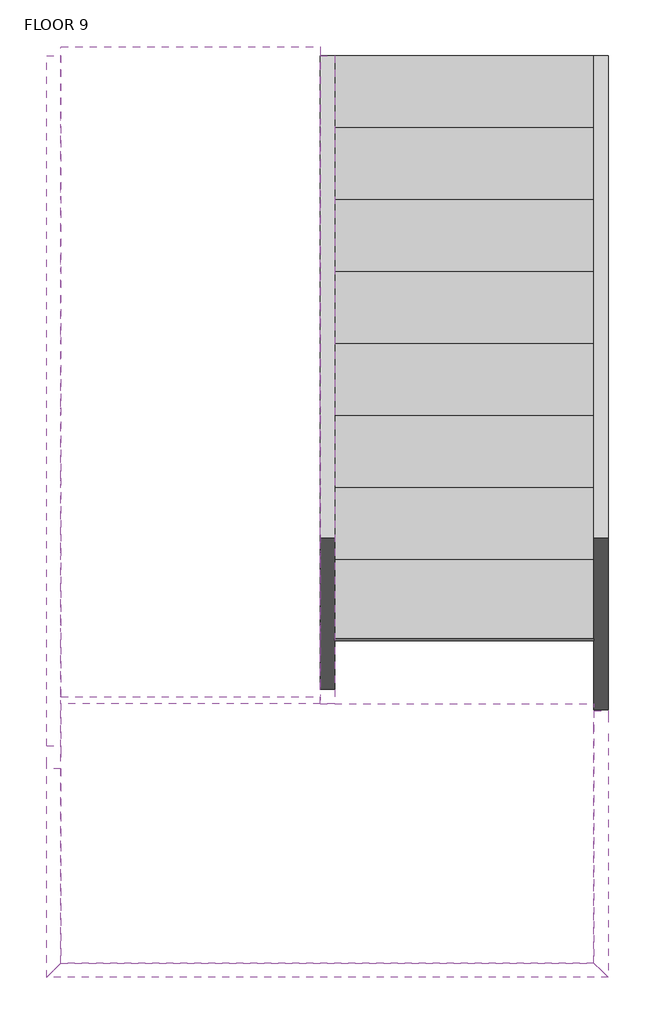
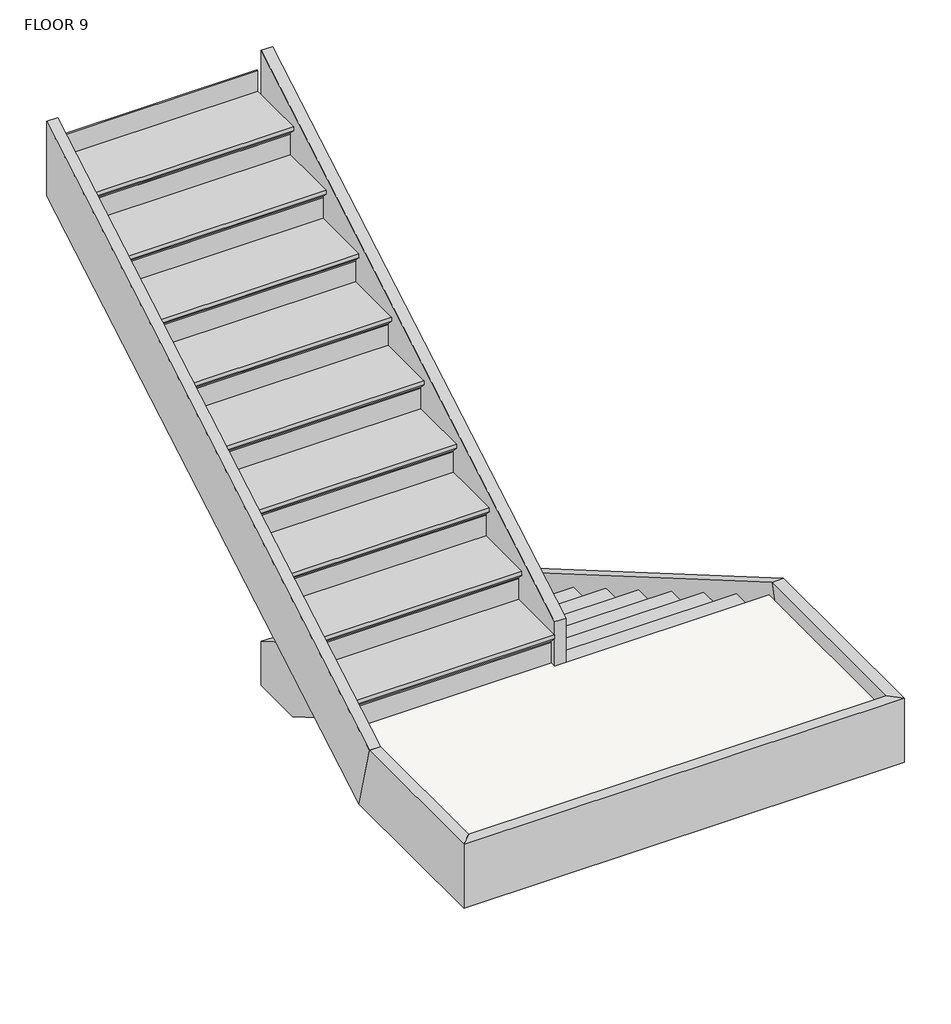
# One storey, incomplete: 7 members, 2 stair flights, 1 slab.
"""IFC4 building model written with IfcOpenShell, lengths in millimetres."""

from ifc_helpers import new_model, si_unit, frame, origin, place, context, project, spatial, polyline, outline, extrude, faceted_brep, transform, mapped, element, save
from components import non_monolithic_landing_daa301cf, stair_flight_c4a53ddb, stair_flight_6c6ce143

model = new_model("IFC4")

# Units and contexts
model_context = context("Model", 3, world=origin())
ifc_project = project(units=[si_unit("LENGTHUNIT", "METRE", prefix="MILLI")], contexts=[model_context])

# Site, building, storey
site = spatial("IfcSite", under=ifc_project)
building = spatial("IfcBuilding", under=site)
storey = spatial("IfcBuildingStorey", under=building, Name="FLOOR 9", Elevation=9544.3725604)

# Members
placement = place(None, origin())
element("IfcMember", 1, ObjectType="Stringer - 2\" Width", at=placement, inside=storey, context=model_context, shape_type="SweptSolid", body=[
    extrude(outline(polyline([(-4241.0593836, 9754.2933656), (-4241.0593836, 9544.3725604), (-4486.3086974, 9544.3725604), (-6633.5807846, 10794.2618174), (-6551.3310691, 11099.0618174), (-4241.0593836, 9754.2933656)])), frame((-3400.7137331, 0.0, 0.0), z_axis=(1.0, 0.0, 0.0), x_axis=(0.0, 1.0, 0.0)), (0.0, 0.0, 1.0), 50.8),
])
element("IfcMember", 2, ObjectType="Stringer - 2\" Width", at=placement, inside=storey, context=model_context, shape_type="SweptSolid", body=[
    extrude(outline(polyline([(-4241.0593836, 9754.2933656), (-4241.0593836, 9544.3725604), (-4486.3086974, 9544.3725604), (-6476.2593836, 10702.6878011), (-6476.2593836, 11055.3639117), (-4241.0593836, 9754.2933656)])), frame((-4365.9137331, 0.0, 0.0), z_axis=(1.0, 0.0, 0.0), x_axis=(0.0, 1.0, 0.0)), (0.0, 0.0, 1.0), 50.8),
])
element("IfcMember", 3, ObjectType="Stringer - 2\" Width", at=placement, inside=storey, context=model_context, shape_type="SweptSolid", body=[
    extrude(outline(polyline([(-6674.5379826, 10794.2618174), (-6756.7876981, 11099.0618174), (-4241.0593836, 12563.4229538), (-4241.0593836, 12210.7468432), (-6674.5379826, 10794.2618174)])), frame((-5331.1137331, 0.0, 0.0), z_axis=(1.0, 0.0, 0.0), x_axis=(0.0, 1.0, 0.0)), (0.0, 0.0, 1.0), 50.8),
])
element("IfcMember", 4, ObjectType="Stringer - 2\" Width", at=placement, inside=storey, context=model_context, shape_type="SweptSolid", body=[
    extrude(outline(polyline([(-6527.0593836, 10880.106512), (-6527.0593836, 11232.7826225), (-4241.0593836, 12563.4229538), (-4241.0593836, 12210.7468432), (-6527.0593836, 10880.106512)])), frame((-4365.9137331, 0.0, 0.0), z_axis=(1.0, 0.0, 0.0), x_axis=(0.0, 1.0, 0.0)), (0.0, 0.0, 1.0), 50.8),
])
element("IfcMember", 5, ObjectType="Stringer - 2\" Width", at=placement, inside=storey, context=model_context, shape_type="Brep", body=[
    faceted_brep([(-5280.3137331, -6756.7876981, 11099.0618174), (-5331.1137331, -6756.7876981, 11099.0618174), (-5331.1137331, -7492.2593836, 11099.0618174), (-5280.3137331, -7441.4593836, 11099.0618174), (-5280.3137331, -6674.5379826, 10794.2618174), (-5280.3137331, -7441.4593836, 10794.2618174), (-5331.1137331, -6674.5379826, 10794.2618174), (-5331.1137331, -7492.2593836, 10794.2618174)], [[[0, 1, 2, 3]], [[4, 0, 3, 5]], [[6, 4, 5, 7]], [[1, 6, 7, 2]], [[1, 0, 4, 6]], [[2, 7, 5, 3]]]),
])
element("IfcMember", 6, ObjectType="Stringer - 2\" Width", at=placement, inside=storey, context=model_context, shape_type="SweptSolid", body=[
    extrude(outline(polyline([(-5331.1137331, -7492.2593836), (-5280.3137331, -7441.4593836), (-3400.7137331, -7441.4593836), (-3349.9137331, -7492.2593836), (-5331.1137331, -7492.2593836)])), frame((0.0, 0.0, 10794.2618174), z_axis=(0.0, 0.0, 1.0), x_axis=(1.0, 0.0, 0.0)), (0.0, 0.0, 1.0), 304.8),
])
element("IfcMember", 7, ObjectType="Stringer - 2\" Width", at=placement, inside=storey, context=model_context, shape_type="Brep", body=[
    faceted_brep([(-3400.7137331, -7441.4593836, 11099.0618174), (-3349.9137331, -7492.2593836, 11099.0618174), (-3349.9137331, -6551.3310691, 11099.0618174), (-3400.7137331, -6551.3310691, 11099.0618174), (-3400.7137331, -7441.4593836, 10794.2618174), (-3400.7137331, -6633.5807846, 10794.2618174), (-3349.9137331, -7492.2593836, 10794.2618174), (-3349.9137331, -6633.5807846, 10794.2618174)], [[[0, 1, 2, 3]], [[4, 0, 3, 5]], [[6, 4, 5, 7]], [[1, 6, 7, 2]], [[1, 0, 4, 6]], [[2, 7, 5, 3]]]),
])

# Slab
non_monolithic_landing_shape = non_monolithic_landing_daa301cf(model_context)
element("IfcSlab", 8, ObjectType="Non-Monolithic Landing", at=placement, inside=storey, context=model_context, shape_type="MappedRepresentation", body=[
    mapped(non_monolithic_landing_shape, transform((0.0, 0.0, 0.0), x_axis=(1.0, 0.0, 0.0), y_axis=(0.0, 1.0, 0.0), z_axis=(0.0, 0.0, 1.0))),
])

# Stair flights
stair_flight_shape = stair_flight_c4a53ddb(model_context)
element("IfcStairFlight", 9, ObjectType="2\" Tread 1\" Nosing 1/4\" Riser", at=placement, inside=storey, context=model_context, shape_type="MappedRepresentation", body=[
    mapped(stair_flight_shape, transform((0.0, 0.0, 0.0), x_axis=(1.0, 0.0, 0.0), y_axis=(0.0, 1.0, 0.0), z_axis=(0.0, 0.0, 1.0))),
])
stair_flight_2_shape = stair_flight_6c6ce143(model_context)
element("IfcStairFlight", 10, ObjectType="2\" Tread 1\" Nosing 1/4\" Riser", at=placement, inside=storey, context=model_context, shape_type="MappedRepresentation", body=[
    mapped(stair_flight_2_shape, transform((0.0, 0.0, 0.0), x_axis=(1.0, 0.0, 0.0), y_axis=(0.0, 1.0, 0.0), z_axis=(0.0, 0.0, 1.0))),
])

save(model, "model.ifc")

# Revit data of these elements
# Elements 1, 2, 3, 4, 5, 6, 7 (IfcMember, "Stringer - 2\" Width")
#   Phase Created = New Construction
# Element 8 (IfcSlab, "Non-Monolithic Landing")
#   Phase Created = New Construction
# Elements 9, 10 (IfcStairFlight, "2\" Tread 1\" Nosing 1/4\" Riser")
#   Phase Created = New Construction
